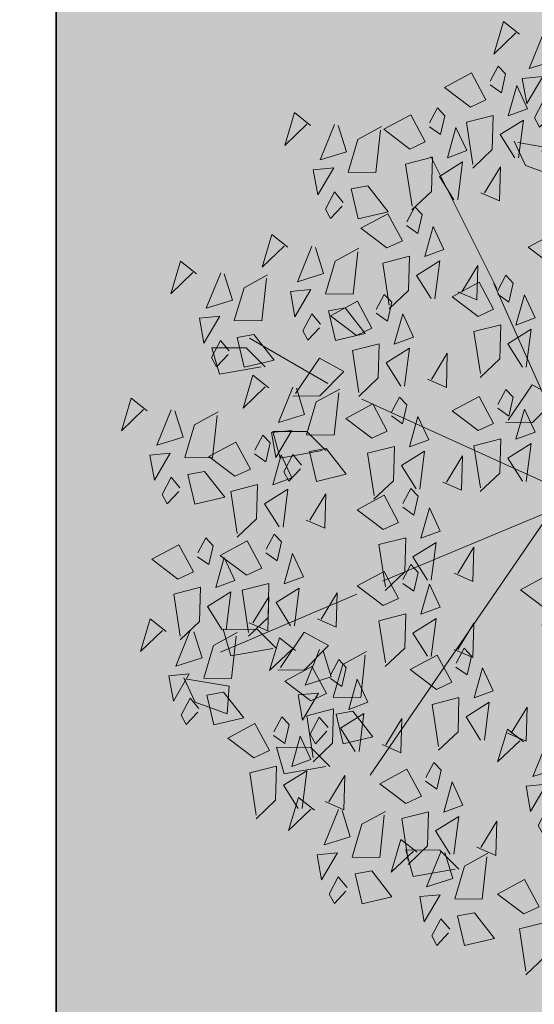
# Model space of a CAD drawing. Units: inches. Extents: x 1704 to 6393, y -157 to 1172.
# Tile 67 of 122: x 1897 to 1913, y 980 to 1010. Entities that reach past the tile are written whole.
import ezdxf

# ---------------------------------------------------------------- set-up
doc = ezdxf.new("R2010")
doc.units = ezdxf.units.IN
doc.header["$MEASUREMENT"] = 0
for name, color, linetype, lineweight in [('A-ANNO-DIMS', 7, 'Continuous', 13), ('C-PROP', 7, 'Continuous', 35), ('L-shrub', 74, 'Continuous', 18)]:
    doc.layers.add(name, color=color, linetype=linetype, lineweight=lineweight)
doc.layers.add('L-HRDS-PATT', color=9, linetype='Continuous', lineweight=13, true_color=0xc5c1ba)
doc.styles.get("Standard").update_dxf_attribs({"font": 'arial.ttf'})
doc.dimstyles.get("Standard").update_dxf_attribs({"dimtxt": 6, "dimasz": 2, "dimexe": 0.18, "dimexo": 0.0625, "dimgap": 0.09, "dimtad": 0, "dimtih": 1, "dimtoh": 1, "dimdec": 1, "dimzin": 0, "dimdsep": 46, "dimlunit": 3, "dimtxsty": 'Standard', "dimblk": 'ARCHTICK', "dimcen": 0.09, "dimadec": 0, "dimazin": 0, "dimtfac": 1, "dimtdec": 1, "dimtofl": 0, "dimtmove": 0, "dimatfit": 3, "dimfxl": 1, "dimtolj": 1, "dimtzin": 0, "dimarcsym": 0})

# ---------------------------------------------------------------- blocks, each defined once
blk = doc.blocks.new('flower shrub 3')
at = {"layer": 'L-shrub'}
for p, q in [((-123.45, 236), (-108.99, 242.75)), ((-109.76, 240.63), (-114.02, 215.74)), ((-130.41, 216.9), (-123.45, 236)), ((71.14, 221.55), (86.95, 226.01)), ((86.95, 226.01), (86.87, 205.67)), ((-114.02, 215.74), (-130.41, 216.9)), ((-96.02, 214.78), (-80.21, 219.24)), ((-80.21, 219.24), (-80.29, 198.91)), ((75.55, 196.68), (71.14, 221.55)), ((-91.61, 189.92), (-96.02, 214.78)), ((86.87, 205.67), (75.54, 194.43)), ((-80.29, 198.91), (-91.62, 187.66)), ((-166.05, 183.2), (-150.24, 187.65)), ((-150.24, 187.65), (-150.32, 167.32)), ((21.44, 185.45), (37.25, 189.91)), ((37.25, 189.91), (37.17, 169.58)), ((-161.64, 158.33), (-166.05, 183.2)), ((-104.33, 170.99), (-104.5, 186.95)), ((-102.88, 185.37), (-81.99, 171.19)), ((25.85, 160.59), (21.44, 185.45)), ((58.31, 161.96), (58.15, 177.93)), ((59.76, 176.34), (80.66, 162.16)), ((-89.82, 156.75), (-104.33, 170.99)), ((-81.99, 171.19), (-89.82, 156.75)), ((37.17, 169.58), (25.84, 158.33)), ((-150.32, 167.32), (-161.65, 156.07)), ((72.82, 147.73), (58.31, 161.96)), ((80.66, 162.16), (72.82, 147.73)), ((-227.04, 106.49), (-211.23, 110.94)), ((-222.63, 81.62), (-227.04, 106.49)), ((-211.23, 110.94), (-211.31, 90.61)), ((-211.31, 90.61), (-222.64, 79.36)), ((42.5, 35.62), (42.33, 51.58)), ((43.95, 50), (64.85, 35.82)), ((195.06, 39.71), (209.52, 46.47)), ((208.75, 44.35), (204.49, 19.45)), ((57.01, 21.38), (42.5, 35.62)), ((64.85, 35.82), (57.01, 21.38)), ((188.1, 20.61), (195.06, 39.71)), ((204.49, 19.45), (188.1, 20.61)), ((184.09, 9.47), (199.9, 13.93)), ((199.9, 13.93), (199.81, -6.4)), ((188.5, -15.39), (184.09, 9.47)), ((218.7, -20.78), (218.53, -4.82)), ((199.81, -6.4), (188.49, -17.65)), ((220.15, -6.4), (241.04, -20.58)), ((233.21, -35.02), (218.7, -20.78)), ((241.04, -20.58), (233.21, -35.02)), ((84.69, -53.7), (100.5, -49.25)), ((100.5, -49.25), (100.42, -69.58)), ((89.1, -78.57), (84.69, -53.7)), ((100.42, -69.58), (89.1, -80.83)), ((-205.99, -97.49), (-206.15, -81.53)), ((-204.54, -83.11), (-183.64, -97.29)), ((-191.47, -111.73), (-205.99, -97.49)), ((-183.64, -97.29), (-191.47, -111.73)), ((-161.53, -112.36), (-145.72, -107.91)), ((-145.72, -107.91), (-145.8, -128.24)), ((-157.12, -137.23), (-161.53, -112.36)), ((-179.93, -131.75), (-165.46, -125)), ((-166.23, -127.12), (-170.5, -152.01)), ((-145.8, -128.24), (-157.13, -139.49)), ((-186.88, -150.86), (-179.93, -131.75)), ((143.42, -141.69), (159.24, -137.24)), ((159.24, -137.24), (159.15, -157.57)), ((147.84, -166.56), (143.42, -141.69)), ((-170.5, -152.01), (-186.88, -150.86)), ((-163.07, -171.95), (-163.23, -155.98)), ((-161.62, -157.57), (-140.72, -171.75)), ((159.15, -157.57), (147.83, -168.82)), ((-148.55, -186.18), (-163.07, -171.95)), ((-140.72, -171.75), (-148.55, -186.18)), ((10.15, -195.84), (25.96, -191.38)), ((25.96, -191.38), (25.88, -211.71)), ((14.56, -220.7), (10.15, -195.84)), ((25.88, -211.71), (14.55, -222.96))]:
    blk.add_line(p, q, dxfattribs=at)
for points in [[(49.51, 264.41), (57.05, 273.94), (37.55, 279.71), (50.15, 266.57)], [(-81.5, 253.13), (-73.97, 262.66), (-93.47, 268.43), (-80.86, 255.29)], [(-50.38, 246.16), (-38.67, 261.64), (-30.06, 245.61), (-46.11, 237.01), (-50.38, 246.16)], [(24.26, 250.7), (23.13, 262.8), (8.21, 260.16), (24.26, 250.7)], [(49.36, 247.98), (33.81, 243.17), (28.98, 258.72), (50, 250.14)], [(-106.76, 239.42), (-107.89, 251.52), (-122.81, 248.88), (-106.76, 239.42)], [(3.73, 245.02), (9.98, 250.22), (-0.21, 255.59), (-5.82, 252.55), (1.56, 245.66)], [(-81.65, 236.7), (-97.21, 231.89), (-102.03, 247.44), (-81.01, 238.86)], [(-84.31, 244.82), (-59.35, 248.66), (-55.26, 232.75), (-75.59, 233.29), (-86.57, 244.88)], [(130.84, 235.08), (138.37, 244.61), (118.87, 250.38), (131.48, 237.24)], [(-127.29, 233.74), (-121.04, 238.94), (-131.23, 244.31), (-136.84, 241.27), (-129.46, 234.38)], [(13.52, 230.35), (-1.79, 218.41), (-5.97, 236.12), (11.75, 240.29), (13.52, 230.35)], [(46.65, 222.9), (21.55, 225.63), (21.7, 242.05), (41.19, 236.28), (48.82, 222.26)], [(-37.14, 234.51), (-41.84, 227.87), (-30.61, 225.31), (-25.97, 229.7), (-34.88, 234.45)], [(-117.5, 219.07), (-132.81, 207.13), (-136.99, 224.84), (-119.27, 229.01), (-117.5, 219.07)], [(-84.36, 211.62), (-109.47, 214.34), (-109.32, 230.77), (-89.83, 225), (-82.2, 210.98)], [(-80.47, 219.88), (-66.68, 228.54), (-58.01, 214.76), (-80.53, 217.63)], [(105.58, 221.37), (104.45, 233.47), (89.53, 230.83), (105.58, 221.37)], [(130.69, 218.65), (115.13, 213.84), (110.31, 229.39), (131.33, 220.81)], [(-55.51, 223.72), (-51.3, 212.33), (-37.56, 218.73), (-55.51, 223.72)], [(10.61, 212.31), (22.33, 227.8), (30.93, 211.77), (14.88, 203.17), (10.61, 212.31)], [(85.05, 215.69), (91.3, 220.89), (81.11, 226.26), (75.5, 223.22), (82.88, 216.33)], [(-156.55, 201.03), (-144.84, 216.52), (-136.23, 200.48), (-152.28, 191.89), (-156.55, 201.03)], [(-59.39, 140.01), (-93.72, 220.83)], [(-48.12, 205.55), (-36.41, 221.03), (-27.8, 205), (-43.85, 196.4), (-48.12, 205.55)], [(-23.32, 210.97), (1.64, 214.81), (5.73, 198.9), (-14.6, 199.45), (-25.58, 211.03)], [(94.84, 201.02), (79.53, 189.08), (75.35, 206.79), (93.07, 210.96), (94.84, 201.02)], [(127.98, 193.57), (102.87, 196.3), (103.02, 212.72), (122.51, 206.95), (130.14, 192.93)], [(-82.06, 204.2), (-57.09, 208.04), (-53, 192.14), (-73.33, 192.68), (-84.31, 204.27)], [(63.07, 192.21), (70.6, 201.74), (51.11, 207.51), (63.71, 194.37)], [(-190.49, 199.69), (-165.52, 203.53), (-161.43, 187.62), (-181.76, 188.17), (-192.74, 199.75)], [(-76.38, 203.98), (-81.2, 192.82), (-60.88, 192.27), (-76.44, 201.72)], [(23.85, 200.67), (19.16, 194.03), (30.38, 191.47), (35.02, 195.86), (26.11, 200.61)], [(65.66, 157.16), (92.63, 203.69)], [(-34.88, 193.9), (-39.58, 187.26), (-28.35, 184.7), (-23.71, 189.09), (-32.62, 193.84)], [(-19.48, 186.04), (-5.68, 194.7), (2.98, 180.92), (-19.54, 183.79)], [(146.65, 180.93), (154.18, 190.46), (134.69, 196.23), (147.29, 183.09)], [(-143.31, 189.39), (-148.01, 182.75), (-136.78, 180.19), (-132.14, 184.58), (-141.05, 189.33)], [(-92.8, 176.42), (-85.27, 185.95), (-104.76, 191.72), (-92.16, 178.58)], [(-78.21, 179.27), (-64.42, 187.93), (-55.75, 174.15), (-78.27, 177.02)], [(5.48, 189.88), (9.7, 178.48), (23.43, 184.88), (5.48, 189.88)], [(37.81, 178.51), (36.68, 190.61), (21.76, 187.96), (37.81, 178.51)], [(-186.64, 174.76), (-172.85, 183.42), (-164.18, 169.64), (-186.7, 172.51)], [(-122.67, 167.19), (-110.95, 182.67), (-102.35, 166.64), (-118.4, 158.05), (-122.67, 167.19)], [(-53.25, 183.11), (-49.04, 171.72), (-35.3, 178.12), (-53.25, 183.11)], [(17.28, 172.82), (23.53, 178.03), (13.34, 183.4), (7.73, 180.35), (15.12, 173.46)], [(62.92, 175.78), (47.36, 170.98), (42.54, 186.52), (63.56, 177.95)], [(218.93, 167.39), (226.47, 176.93), (206.97, 182.7), (219.58, 169.56)], [(-187.68, 165.14), (-180.14, 174.67), (-199.64, 180.44), (-187.04, 167.3)], [(-161.68, 178.6), (-157.47, 167.2), (-143.73, 173.6), (-161.68, 178.6)], [(121.39, 167.23), (120.26, 179.33), (105.34, 176.68), (121.39, 167.23)], [(-156.6, 165.85), (-131.64, 169.69), (-127.55, 153.78), (-147.87, 154.33), (-158.86, 165.91)], [(-118.06, 162.71), (-119.19, 174.81), (-134.1, 172.17), (-118.06, 162.71)], [(-92.95, 159.99), (-108.51, 155.18), (-113.33, 170.73), (-92.31, 162.15)], [(-15.39, 170.13), (-20.21, 158.98), (0.12, 158.43), (-15.45, 167.88)], [(60.21, 150.7), (35.1, 153.43), (35.25, 169.85), (54.74, 164.09), (62.37, 150.06)], [(100.86, 161.54), (107.11, 166.75), (96.92, 172.11), (91.31, 169.07), (98.7, 162.18)], [(146.5, 164.5), (130.94, 159.7), (126.12, 175.24), (147.14, 166.67)], [(-138.59, 157.03), (-132.33, 162.23), (-142.52, 167.6), (-148.14, 164.56), (-140.75, 157.67)], [(27.08, 158.16), (11.76, 146.22), (7.58, 163.93), (25.31, 168.09), (27.08, 158.16)], [(193.68, 153.69), (192.55, 165.79), (177.63, 163.15), (193.68, 153.69)], [(-212.93, 151.43), (-214.06, 163.53), (-228.98, 160.89), (-212.93, 151.43)], [(-187.82, 148.71), (-203.38, 143.9), (-208.21, 159.45), (-187.18, 150.87)], [(-182.55, 158.85), (-187.37, 147.7), (-167.05, 147.15), (-182.61, 156.6)], [(-74.12, 163.36), (-78.94, 152.21), (-58.62, 151.66), (-74.18, 161.11)], [(143.79, 139.42), (118.68, 142.15), (118.83, 158.57), (138.33, 152.8), (145.96, 138.78)], [(173.15, 148), (179.4, 153.21), (169.21, 158.58), (163.6, 155.53), (170.98, 148.64)], [(218.79, 150.97), (203.23, 146.16), (198.41, 161.7), (219.43, 153.13)], [(-233.46, 145.75), (-227.21, 150.95), (-237.4, 156.32), (-243.01, 153.28), (-235.63, 146.39)], [(-128.79, 142.36), (-144.1, 130.42), (-148.29, 148.13), (-130.56, 152.3), (-128.79, 142.36)], [(-95.66, 134.91), (-120.77, 137.64), (-120.62, 154.06), (-101.12, 148.29), (-93.49, 134.27)], [(-109.42, 155.55), (-114.12, 148.9), (-102.89, 146.34), (-98.26, 150.73), (-107.17, 155.49)], [(110.66, 146.88), (95.35, 134.94), (91.16, 152.64), (108.89, 156.81), (110.66, 146.88)], [(94.19, 140.12), (105.91, 155.6), (114.51, 139.57), (98.46, 130.97), (94.19, 140.12)], [(-152.75, 140.92), (-138.96, 149.57), (-130.29, 135.8), (-152.82, 138.66)], [(33.2, 131.09), (44.92, 146.57), (53.52, 130.54), (37.47, 121.95), (33.2, 131.09)], [(-223.67, 131.08), (-238.98, 119.14), (-243.16, 136.85), (-225.44, 141.02), (-223.67, 131.08)], [(-190.53, 123.63), (-215.64, 126.35), (-215.49, 142.78), (-196, 137.01), (-188.37, 122.99)], [(-127.79, 144.76), (-123.58, 133.36), (-109.85, 139.76), (-127.79, 144.76)], [(60.26, 138.78), (85.22, 142.62), (89.31, 126.71), (68.99, 127.26), (58, 138.84)], [(182.94, 133.34), (167.63, 121.4), (163.45, 139.11), (181.17, 143.27), (182.94, 133.34)], [(216.08, 125.89), (190.97, 128.61), (191.12, 145.04), (210.61, 139.27), (218.24, 125.25)], [(-66.19, 124.32), (-54.48, 139.81), (-45.87, 123.78), (-61.92, 115.18), (-66.19, 124.32)], [(-21.02, 124.32), (-9.3, 139.81), (-0.69, 123.78), (-16.74, 115.18), (-21.02, 124.32)], [(-2.54, 7.13), (56.31, 136.92)], [(146.15, 122.07), (157.86, 137.55), (166.47, 121.52), (150.42, 112.92), (146.15, 122.07)], [(-9.89, 24.27), (-166.82, 132.02)], [(-0.73, 129.75), (24.23, 133.59), (28.32, 117.68), (7.99, 118.23), (-2.99, 129.81)], [(-183.66, 110.79), (-171.94, 126.27), (-163.34, 110.24), (-179.39, 101.64), (-183.66, 110.79)], [(-148.66, 125.01), (-153.48, 113.86), (-133.16, 113.31), (-148.73, 122.75)], [(-100.13, 122.98), (-75.17, 126.82), (-71.08, 110.91), (-91.4, 111.46), (-102.39, 123.04)], [(-54.95, 122.98), (-29.99, 126.82), (-25.9, 110.91), (-46.22, 111.46), (-57.21, 123.04)], [(-2.54, 7.13), (-51.58, 124.68)], [(107.43, 128.47), (102.74, 121.83), (113.97, 119.27), (118.6, 123.66), (109.69, 128.41)], [(112.21, 120.73), (137.17, 124.57), (141.26, 108.66), (120.94, 109.21), (109.96, 120.79)], [(204.88, 108.53), (216.6, 124.01), (225.2, 107.98), (209.15, 99.39), (204.88, 108.53)], [(-212.52, 104.22), (-204.99, 113.75), (-224.49, 119.52), (-211.88, 106.38)], [(46.44, 119.45), (41.74, 112.81), (52.97, 110.25), (57.61, 114.63), (48.7, 119.39)], [(64.1, 113.85), (77.9, 122.5), (86.56, 108.73), (64.04, 111.59)], [(89.07, 117.69), (93.28, 106.29), (107.01, 112.69), (89.07, 117.69)], [(-217.59, 109.45), (-192.63, 113.29), (-188.54, 97.38), (-208.86, 97.93), (-219.85, 109.51)], [(-52.95, 112.68), (-57.65, 106.04), (-46.42, 103.48), (-41.78, 107.87), (-50.69, 112.62)], [(-7.77, 112.68), (-12.47, 106.04), (-1.24, 103.48), (3.4, 107.87), (-5.51, 112.62)], [(3.11, 104.82), (16.91, 113.48), (25.57, 99.7), (3.05, 102.57)], [(-115.89, 92.74), (-104.17, 108.22), (-95.57, 92.19), (-111.62, 83.59), (-115.89, 92.74)], [(-96.28, 98.05), (-82.49, 106.71), (-73.82, 92.93), (-96.34, 95.8)], [(-51.1, 98.05), (-37.31, 106.71), (-28.64, 92.93), (-51.16, 95.8)], [(28.07, 108.66), (32.29, 97.26), (46.02, 103.66), (28.07, 108.66)], [(159.39, 110.43), (154.69, 103.78), (165.92, 101.22), (170.56, 105.61), (161.65, 110.36)], [(170.95, 107.19), (195.91, 111.03), (200, 95.12), (179.67, 95.67), (168.69, 107.25)], [(-237.78, 90.52), (-238.91, 102.62), (-253.83, 99.97), (-237.78, 90.52)], [(-71.32, 101.89), (-67.11, 90.49), (-53.38, 96.89), (-71.32, 101.89)], [(-26.14, 101.89), (-21.93, 90.49), (-8.2, 96.89), (-26.14, 101.89)], [(116.06, 95.8), (129.85, 104.45), (138.52, 90.68), (116, 93.54)], [(141.02, 99.64), (145.23, 88.24), (158.96, 94.64), (141.02, 99.64)], [(-258.31, 84.83), (-252.06, 90.04), (-262.25, 95.41), (-267.86, 92.36), (-260.48, 85.47)], [(-212.67, 87.79), (-228.23, 82.99), (-233.05, 98.53), (-212.03, 89.96)], [(-170.42, 99.14), (-175.11, 92.5), (-163.88, 89.94), (-159.25, 94.33), (-168.16, 99.08)], [(-149.82, 91.4), (-124.86, 95.24), (-120.77, 79.33), (-141.1, 79.88), (-152.08, 91.46)], [(68.19, 97.94), (63.37, 86.78), (83.7, 86.23), (68.13, 95.68)], [(122.05, 56.75), (200.52, 95.93)], [(218.12, 96.89), (213.42, 90.24), (224.65, 87.68), (229.29, 92.07), (220.38, 96.83)], [(-213.75, 84.52), (-199.95, 93.17), (-191.29, 79.4), (-213.81, 82.26)], [(-188.78, 88.36), (-184.57, 76.96), (-170.84, 83.36), (-188.78, 88.36)], [(7.2, 88.91), (2.38, 77.76), (22.71, 77.21), (7.14, 86.66)], [(174.79, 82.26), (188.58, 90.91), (197.25, 77.14), (174.73, 80)], [(229.73, 72.43), (241.44, 87.91), (250.05, 71.88), (234, 63.29), (229.73, 72.43)], [(-215.38, 62.71), (-240.49, 65.44), (-240.34, 81.86), (-220.85, 76.1), (-213.22, 62.07)], [(-92.19, 82.14), (-97.01, 70.99), (-76.69, 70.44), (-92.25, 79.89)], [(-47.01, 82.14), (-51.83, 70.99), (-31.51, 70.44), (-47.07, 79.89)], [(37.72, 67.92), (49.43, 83.4), (58.04, 67.37), (41.99, 58.78), (37.72, 67.92)], [(105.49, 67.92), (117.2, 83.4), (125.81, 67.37), (109.76, 58.78), (105.49, 67.92)], [(199.75, 86.1), (203.97, 74.7), (217.7, 81.1), (199.75, 86.1)], [(-248.51, 70.17), (-263.83, 58.23), (-268.01, 75.94), (-250.29, 80.1), (-248.51, 70.17)], [(-102.65, 81.1), (-107.35, 74.45), (-96.12, 71.89), (-91.48, 76.28), (-100.39, 81.03)], [(120.15, 79.89), (115.33, 68.73), (135.65, 68.18), (120.09, 77.63)], [(-145.98, 66.47), (-132.19, 75.12), (-123.52, 61.35), (-146.04, 64.21)], [(-121.02, 70.31), (-116.8, 58.91), (-103.07, 65.31), (-121.02, 70.31)], [(3.78, 66.58), (28.75, 70.42), (32.84, 54.51), (12.51, 55.06), (1.53, 66.64)], [(71.55, 66.58), (96.51, 70.42), (100.6, 54.51), (80.28, 55.06), (69.29, 66.64)], [(195.79, 71.09), (220.76, 74.93), (224.85, 59.02), (204.52, 59.57), (193.54, 71.15)], [(-209.66, 68.61), (-214.48, 57.45), (-194.15, 56.9), (-209.72, 66.35)], [(178.88, 66.35), (174.06, 55.2), (194.39, 54.65), (178.82, 64.09)], [(9.72, 7.13), (124.97, 58.56)], [(242.97, 60.79), (238.27, 54.15), (249.5, 51.59), (254.14, 55.97), (245.23, 60.73)], [(273.15, 43.3), (280.68, 52.84), (261.19, 58.61), (273.79, 45.47)], [(-249.17, 40.85), (-237.45, 56.33), (-228.85, 40.3), (-244.9, 31.7), (-249.17, 40.85)], [(-147.01, 41.05), (-139.48, 50.58), (-158.98, 56.35), (-146.37, 43.21)], [(50.96, 56.28), (46.26, 49.63), (57.49, 47.07), (62.13, 51.46), (53.22, 56.22)], [(118.73, 56.28), (114.03, 49.63), (125.26, 47.07), (129.9, 51.46), (120.99, 56.22)], [(199.64, 46.16), (213.43, 54.82), (222.1, 41.04), (199.58, 43.91)], [(-141.89, 50.56), (-146.71, 39.4), (-126.38, 38.85), (-141.95, 48.3)], [(7.63, 41.65), (21.42, 50.3), (30.09, 36.53), (7.57, 39.39)], [(75.4, 41.65), (89.19, 50.3), (97.86, 36.53), (75.34, 39.39)], [(224.6, 50), (228.81, 38.6), (242.55, 45), (224.6, 50)], [(-283.1, 39.51), (-258.14, 43.35), (-254.05, 27.44), (-274.37, 27.98), (-285.36, 39.57)], [(-68.45, 27.31), (-56.74, 42.79), (-48.13, 26.76), (-64.18, 18.17), (-68.45, 27.31)], [(32.59, 45.49), (36.8, 34.09), (50.54, 40.49), (32.59, 45.49)], [(100.36, 45.49), (104.57, 34.09), (118.3, 40.49), (100.36, 45.49)], [(247.89, 29.6), (246.76, 41.7), (231.84, 39.06), (247.89, 29.6)], [(-172.27, 27.35), (-173.4, 39.44), (-188.32, 36.8), (-172.27, 27.35)], [(-147.16, 24.62), (-162.72, 19.81), (-167.54, 35.36), (-146.52, 26.78)], [(134.85, 22.8), (146.57, 38.28), (155.17, 22.25), (139.12, 13.65), (134.85, 22.8)], [(273, 26.88), (257.44, 22.07), (252.62, 37.61), (273.64, 29.04)], [(-192.8, 21.66), (-186.55, 26.86), (-196.74, 32.23), (-202.35, 29.19), (-194.97, 22.3)], [(-102.39, 25.97), (-77.43, 29.81), (-73.34, 13.9), (-93.66, 14.45), (-104.64, 26.03)], [(203.73, 30.25), (198.91, 19.1), (219.23, 18.55), (203.67, 28)], [(227.36, 23.91), (233.62, 29.12), (223.43, 34.49), (217.81, 31.44), (225.2, 24.55)], [(-235.92, 29.2), (-240.62, 22.56), (-229.39, 20), (-224.76, 24.39), (-233.67, 29.14)], [(11.72, 25.74), (6.9, 14.58), (27.22, 14.04), (11.66, 23.48)], [(14.63, 7.13), (137.23, 26.72)], [(79.49, 25.74), (74.67, 14.58), (94.99, 14.04), (79.43, 23.48)], [(100.92, 21.46), (125.88, 25.3), (129.97, 9.39), (109.65, 9.94), (98.66, 21.52)], [(-279.26, 14.57), (-265.46, 23.23), (-256.8, 9.45), (-279.32, 12.32)], [(-254.29, 18.41), (-250.08, 7.02), (-236.35, 13.42), (-254.29, 18.41)], [(-149.87, -0.46), (-174.98, 2.27), (-174.83, 18.69), (-155.34, 12.92), (-147.71, -1.1)], [(-113.13, 7.2), (-105.6, 16.74), (-125.09, 22.51), (-112.49, 9.37)], [(92.43, 4.95), (99.97, 14.48), (80.47, 20.25), (93.07, 7.11)], [(237.16, 9.25), (221.85, -2.69), (217.66, 15.02), (235.39, 19.19), (237.16, 9.25)], [(270.29, 1.8), (245.18, 4.52), (245.33, 20.95), (264.83, 15.18), (272.46, 1.16)], [(-183.01, 6.99), (-198.32, -4.95), (-202.5, 12.76), (-184.78, 16.93), (-183.01, 6.99)], [(-138.39, -6.5), (-139.52, 5.6), (-154.26, 11.88), (-138.39, -6.5)], [(-55.21, 15.67), (-59.91, 9.02), (-48.68, 6.46), (-44.04, 10.85), (-52.95, 15.61)], [(168.74, 0.24), (180.45, 15.72), (189.06, -0.31), (173.01, -8.91), (168.74, 0.24)], [(-98.54, 1.04), (-84.75, 9.69), (-76.08, -4.08), (-98.6, -1.22)], [(148.1, 11.15), (143.4, 4.51), (154.63, 1.95), (159.26, 6.34), (150.35, 11.09)], [(-7.44, 4.68), (-201.15, -54.09)], [(-113.28, -9.22), (-128.84, -14.03), (-133.66, 1.52), (-112.64, -7.06)], [(-73.58, 4.88), (-69.37, -6.52), (-55.64, -0.12), (-73.58, 4.88)], [(14.63, 4.68), (156.84, -137.36)], [(67.18, -8.75), (66.05, 3.35), (51.13, 0.7), (67.18, -8.75)], [(104.77, -3.47), (118.56, 5.18), (127.22, -8.59), (104.7, -5.73)], [(129.73, 0.37), (133.94, -11.03), (147.67, -4.63), (129.73, 0.37)], [(134.8, -1.11), (159.76, 2.73), (163.85, -13.17), (143.53, -12.63), (132.54, -1.04)], [(-275.17, -1.33), (-279.99, -12.49), (-259.66, -13.04), (-275.23, -3.59)], [(-197.21, -15.56), (-185.5, -0.08), (-176.89, -16.11), (-192.94, -24.7), (-197.21, -15.56)], [(-2.54, -0.22), (-181.53, -98.18)], [(-158.92, -12.19), (-152.66, -6.98), (-162.85, -1.61), (-168.47, -4.65), (-161.08, -11.54)], [(-2.54, -5.12), (-51.58, -205.93)], [(-41.35, -15.56), (-29.63, -0.08), (-21.02, -16.11), (-37.07, -24.7), (-41.35, -15.56)], [(46.65, -14.44), (52.9, -9.23), (42.71, -3.87), (37.1, -6.91), (44.48, -13.8)], [(92.28, -11.48), (76.73, -16.28), (71.9, -0.74), (92.92, -9.31)], [(7.27, -10.01), (132.32, -196.13)], [(181.98, -11.41), (177.28, -18.05), (188.51, -20.61), (193.15, -16.22), (184.24, -11.47)], [(223.45, -26.64), (230.99, -17.1), (211.49, -11.33), (224.09, -24.47)], [(-231.15, -16.9), (-206.18, -13.06), (-202.09, -28.97), (-222.42, -28.42), (-233.4, -16.84)], [(-149.12, -26.85), (-164.43, -38.79), (-168.62, -21.08), (-150.89, -16.91), (-149.12, -26.85)], [(-115.99, -34.3), (-141.1, -31.58), (-140.95, -15.15), (-121.45, -20.92), (-113.82, -34.94)], [(-94.45, -14.87), (-99.27, -26.03), (-78.95, -26.58), (-94.51, -17.13)], [(-75.28, -16.9), (-50.32, -13.06), (-46.23, -28.97), (-66.55, -28.42), (-77.54, -16.84)], [(89.57, -36.56), (64.47, -33.83), (64.62, -17.41), (84.11, -23.18), (91.74, -37.2)], [(138.65, -26.04), (152.44, -17.38), (161.11, -31.16), (138.59, -28.29)], [(56.44, -29.1), (41.13, -41.04), (36.95, -23.34), (54.67, -19.17), (56.44, -29.1)], [(108.86, -19.38), (104.03, -30.54), (124.36, -31.09), (108.79, -21.64)], [(163.61, -22.2), (167.82, -33.59), (181.55, -27.19), (163.61, -22.2)], [(-183.97, -27.2), (-188.67, -33.84), (-177.44, -36.4), (-172.8, -32.02), (-181.71, -27.26)], [(-28.1, -27.2), (-32.8, -33.84), (-21.57, -36.4), (-16.93, -32.02), (-25.84, -27.26)], [(55.85, -28.96), (171.09, -41.21)], [(198.2, -40.34), (197.06, -28.24), (182.15, -30.88), (198.2, -40.34)], [(-227.3, -41.83), (-213.51, -33.17), (-204.84, -46.95), (-227.36, -44.08)], [(-71.43, -41.83), (-57.64, -33.17), (-48.97, -46.95), (-71.49, -44.08)], [(37.72, -47.14), (49.43, -31.66), (58.04, -47.69), (41.99, -56.29), (37.72, -47.14)], [(223.3, -43.06), (207.75, -47.87), (202.92, -32.33), (223.94, -40.9)], [(-202.34, -37.99), (-198.13, -49.39), (-184.4, -42.99), (-202.34, -37.99)], [(-124.93, -51.66), (-113.21, -36.17), (-104.6, -52.2), (-120.65, -60.8), (-124.93, -51.66)], [(-46.47, -37.99), (-42.26, -49.39), (-28.53, -42.99), (-46.47, -37.99)], [(-18.76, -53.91), (-7.04, -38.43), (1.57, -54.46), (-14.48, -63.06), (-18.76, -53.91)], [(119.54, -51.46), (127.07, -41.92), (107.58, -36.15), (120.18, -49.29)], [(177.67, -46.03), (183.92, -40.82), (173.73, -35.45), (168.12, -38.5), (175.5, -45.39)], [(-151.53, -58.22), (-144, -48.69), (-163.49, -42.92), (-150.89, -56.06)], [(3.78, -48.48), (28.75, -44.64), (32.84, -60.55), (12.51, -60.01), (1.53, -48.42)], [(142.74, -41.95), (137.92, -53.1), (158.24, -53.65), (142.68, -44.2)], [(-158.86, -53), (-133.9, -49.16), (-129.81, -65.07), (-150.13, -64.52), (-161.12, -52.94)], [(-52.69, -55.25), (-27.73, -51.41), (-23.64, -67.32), (-43.96, -66.77), (-54.95, -55.19)], [(187.46, -60.69), (172.15, -72.63), (167.97, -54.92), (185.69, -50.76), (187.46, -60.69)], [(220.59, -68.14), (195.49, -65.42), (195.64, -48.99), (215.13, -54.76), (222.76, -68.78)], [(266.37, -67.25), (273.91, -57.71), (254.41, -51.94), (267.01, -65.08)], [(-223.21, -57.74), (-228.03, -68.89), (-207.71, -69.44), (-223.27, -59.99)], [(-67.34, -57.74), (-72.16, -68.89), (-51.84, -69.44), (-67.4, -59.99)], [(94.28, -65.16), (93.15, -53.06), (78.24, -55.7), (94.28, -65.16)], [(119.39, -67.88), (103.83, -72.69), (99.01, -57.14), (120.03, -65.72)], [(204.88, -69.71), (216.6, -54.22), (225.2, -70.25), (209.15, -78.85), (204.88, -69.71)], [(-176.79, -71.93), (-177.92, -59.83), (-192.84, -62.47), (-176.79, -71.93)], [(-151.68, -74.65), (-167.24, -79.46), (-172.06, -63.91), (-151.04, -72.49)], [(-111.68, -63.3), (-116.38, -69.94), (-105.15, -72.5), (-100.51, -68.11), (-109.42, -63.36)], [(50.96, -58.79), (46.26, -65.43), (57.49, -67.99), (62.13, -63.6), (53.22, -58.85)], [(73.75, -70.85), (80.01, -65.64), (69.82, -60.27), (64.2, -63.31), (71.59, -70.2)], [(-197.32, -77.61), (-191.07, -72.41), (-201.26, -67.04), (-206.87, -70.08), (-199.48, -76.97)], [(-155.01, -77.93), (-141.22, -69.27), (-132.55, -83.05), (-155.07, -80.18)], [(-5.51, -65.55), (-10.21, -72.2), (1.02, -74.76), (5.66, -70.37), (-3.25, -65.62)], [(7.63, -73.42), (21.42, -64.76), (30.09, -78.54), (7.57, -75.67)], [(32.59, -69.58), (36.8, -80.97), (50.54, -74.57), (32.59, -69.58)], [(170.95, -71.05), (195.91, -67.21), (200, -83.12), (179.67, -82.57), (168.69, -70.99)], [(241.12, -80.95), (239.98, -68.85), (225.07, -71.49), (241.12, -80.95)], [(-130.05, -74.09), (-125.84, -85.49), (-112.11, -79.09), (-130.05, -74.09)], [(-115.89, -90.01), (-104.17, -74.53), (-95.57, -90.56), (-111.62, -99.15), (-115.89, -90.01)], [(-48.84, -80.18), (-35.05, -71.53), (-26.38, -85.3), (-48.9, -82.44)], [(83.55, -85.51), (68.24, -97.45), (64.06, -79.74), (81.78, -75.57), (83.55, -85.51)], [(116.68, -92.96), (91.57, -90.24), (91.72, -73.81), (111.22, -79.58), (118.85, -93.6)], [(116.78, -90.01), (128.5, -74.53), (137.1, -90.56), (121.05, -99.15), (116.78, -90.01)], [(266.22, -83.67), (250.67, -88.48), (245.84, -72.94), (266.86, -81.51)], [(-154.39, -99.73), (-179.5, -97), (-179.35, -80.58), (-159.85, -86.35), (-152.23, -100.37)], [(-49.88, -94.32), (-42.35, -84.79), (-61.84, -79.02), (-49.24, -92.16)], [(-23.88, -76.34), (-19.67, -87.74), (-5.94, -81.34), (-23.88, -76.34)], [(220.59, -86.64), (226.84, -81.43), (216.65, -76.06), (211.04, -79.11), (218.42, -86)], [(218.12, -81.35), (213.42, -87.99), (224.65, -90.55), (229.29, -86.16), (220.38, -81.41)], [(-196.71, -101.09), (-189.18, -91.56), (-208.67, -85.79), (-196.07, -98.93)], [(-187.52, -92.28), (-202.84, -104.22), (-207.02, -86.51), (-189.29, -82.34), (-187.52, -92.28)], [(-149.82, -91.35), (-124.86, -87.51), (-120.77, -103.42), (-141.1, -102.87), (-152.08, -91.29)], [(82.85, -91.35), (107.81, -87.51), (111.9, -103.42), (91.58, -102.87), (80.59, -91.29)], [(174.79, -95.98), (188.58, -87.32), (197.25, -101.1), (174.73, -98.23)], [(-12.8, -148.96), (-20.16, -90.19)], [(11.72, -89.32), (6.9, -100.48), (27.22, -101.03), (11.66, -91.58)], [(62.57, -103.55), (74.28, -88.07), (82.89, -104.1), (66.84, -112.69), (62.57, -103.55)], [(199.75, -92.14), (203.97, -103.54), (217.7, -97.14), (199.75, -92.14)], [(230.38, -101.3), (215.07, -113.24), (210.89, -95.53), (228.61, -91.37), (230.38, -101.3)], [(263.51, -108.75), (238.41, -106.03), (238.56, -89.6), (258.05, -95.37), (265.68, -109.39)], [(-150.92, -93.84), (-155.74, -104.99), (-135.42, -105.54), (-150.98, -96.09)], [(-75.14, -108.02), (-76.27, -95.92), (-91.18, -98.57), (-75.14, -108.02)], [(-44.75, -96.09), (-49.57, -107.25), (-29.25, -107.8), (-44.81, -98.35)], [(-221.97, -114.79), (-223.1, -102.69), (-238.02, -105.34), (-221.97, -114.79)], [(-102.65, -101.65), (-107.35, -108.3), (-96.12, -110.86), (-91.48, -106.47), (-100.39, -101.71)], [(-95.67, -113.71), (-89.41, -108.5), (-99.6, -103.14), (-105.22, -106.18), (-97.83, -113.07)], [(-50.03, -110.75), (-65.59, -115.56), (-70.41, -100.01), (-49.39, -108.58)], [(28.63, -104.89), (53.59, -101.05), (57.68, -116.96), (37.36, -116.41), (26.37, -104.83)], [(70.56, -104.88), (75.47, -144.06)], [(130.02, -101.65), (125.33, -108.3), (136.56, -110.86), (141.19, -106.47), (132.28, -101.71)], [(182.29, -117.08), (194.01, -101.6), (202.61, -117.63), (186.56, -126.23), (182.29, -117.08)], [(-242.5, -120.48), (-236.24, -115.27), (-246.44, -109.9), (-252.05, -112.95), (-244.66, -119.84)], [(-196.86, -117.52), (-212.42, -122.32), (-217.24, -106.78), (-196.22, -115.35)], [(-145.98, -116.28), (-132.19, -107.63), (-123.52, -121.4), (-146.04, -118.54)], [(86.69, -116.28), (100.49, -107.63), (109.15, -121.4), (86.63, -118.54)], [(-121.02, -112.44), (-116.8, -123.84), (-103.07, -117.44), (-121.02, -112.44)], [(-52.74, -135.83), (-77.85, -133.1), (-77.7, -116.68), (-58.2, -122.45), (-50.57, -136.47)], [(75.81, -115.19), (71.11, -121.83), (82.34, -124.39), (86.98, -120.01), (78.07, -115.25)], [(111.65, -112.44), (115.87, -123.84), (129.6, -117.44), (111.65, -112.44)], [(148.36, -118.43), (173.32, -114.59), (177.41, -130.49), (157.08, -129.95), (146.1, -118.36)], [(178.88, -111.89), (174.06, -123.04), (194.39, -123.59), (178.82, -114.14)], [(-181.4, -137.39), (-169.68, -121.91), (-161.08, -137.94), (-177.13, -146.53), (-181.4, -137.39)], [(-85.87, -128.38), (-101.18, -140.31), (-105.37, -122.61), (-87.64, -118.44), (-85.87, -128.38)], [(-0.69, -135.13), (11.03, -119.65), (19.64, -135.68), (3.59, -144.28), (-0.69, -135.13)], [(32.48, -129.82), (46.27, -121.16), (54.94, -134.94), (32.42, -132.07)], [(151.17, -134.93), (158.7, -125.4), (139.2, -119.63), (151.81, -132.77)], [(-232.7, -135.14), (-248.01, -147.08), (-252.2, -129.38), (-234.47, -125.21), (-232.7, -135.14)], [(-199.57, -142.6), (-224.68, -139.87), (-224.53, -123.45), (-205.03, -129.21), (-197.4, -143.24)], [(57.44, -125.98), (61.65, -137.38), (75.38, -130.98), (57.44, -125.98)], [(-141.89, -132.19), (-146.71, -143.35), (-126.38, -143.9), (-141.95, -134.45)], [(-63.94, -146.41), (-52.22, -130.93), (-43.61, -146.96), (-59.66, -155.56), (-63.94, -146.41)], [(-34.62, -136.47), (-9.66, -132.63), (-5.57, -148.54), (-25.89, -148), (-36.88, -136.41)], [(90.78, -132.19), (85.96, -143.35), (106.29, -143.9), (90.72, -134.45)], [(195.53, -128.73), (190.83, -135.37), (202.06, -137.93), (206.7, -133.54), (197.79, -128.79)], [(-215.33, -138.73), (-190.37, -134.89), (-186.28, -150.8), (-206.61, -150.25), (-217.59, -138.67)], [(125.91, -148.63), (124.78, -136.54), (109.86, -139.18), (125.91, -148.63)], [(152.2, -143.36), (166, -134.7), (174.66, -148.48), (152.14, -145.61)], [(177.16, -139.52), (181.38, -150.91), (195.11, -144.51), (177.16, -139.52)], [(-97.87, -147.76), (-72.91, -143.92), (-68.82, -159.82), (-89.14, -159.28), (-100.13, -147.69)], [(36.57, -145.73), (31.75, -156.88), (52.07, -157.43), (36.51, -147.98)], [(105.38, -154.32), (111.63, -149.12), (101.44, -143.75), (95.83, -146.79), (103.21, -153.68)], [(151.02, -151.36), (135.46, -156.17), (130.64, -140.62), (151.66, -149.2)], [(-168.16, -149.03), (-172.86, -155.68), (-161.63, -158.24), (-156.99, -153.85), (-165.9, -149.09)], [(-12.34, -147.15), (-0.08, -242.66)], [(12.56, -146.78), (7.86, -153.42), (19.09, -155.98), (23.73, -151.59), (14.82, -146.84)], [(-211.49, -163.66), (-197.69, -155.01), (-189.03, -168.78), (-211.55, -165.92)], [(-30.77, -161.41), (-16.98, -152.75), (-8.31, -166.53), (-30.83, -163.66)], [(-5.81, -157.57), (-1.6, -168.96), (12.13, -162.56), (-5.81, -157.57)], [(148.31, -176.44), (123.2, -173.71), (123.35, -157.29), (142.84, -163.06), (150.47, -177.08)], [(-186.53, -159.82), (-182.31, -171.22), (-168.58, -164.82), (-186.53, -159.82)], [(-117.65, -177.8), (-110.11, -168.26), (-129.61, -162.5), (-117.01, -175.64)], [(-50.69, -158.06), (-55.39, -164.7), (-44.16, -167.26), (-39.52, -162.87), (-48.43, -158.12)], [(56.29, -177.8), (63.82, -168.26), (44.33, -162.5), (56.93, -175.64)], [(115.18, -168.99), (99.86, -180.93), (95.68, -163.22), (113.4, -159.05), (115.18, -168.99)], [(156.29, -159.27), (151.47, -170.42), (171.8, -170.97), (156.23, -161.52)], [(-94.02, -172.69), (-80.23, -164.03), (-71.56, -177.81), (-94.08, -174.94)], [(-69.06, -168.85), (-64.85, -180.24), (-51.12, -173.84), (-69.06, -168.85)], [(176.01, -186.82), (183.55, -177.29), (164.05, -171.52), (176.66, -184.66)], [(-207.4, -179.57), (-212.22, -190.73), (-191.89, -191.27), (-207.46, -181.83)], [(-142.9, -191.5), (-144.04, -179.4), (-158.95, -182.05), (-142.9, -191.5)], [(-50.38, -193.79), (-38.67, -178.31), (-30.06, -194.34), (-46.11, -202.94), (-50.38, -193.79)], [(-26.68, -177.31), (-31.5, -188.47), (-11.18, -189.02), (-26.74, -179.57)], [(31.03, -191.5), (29.9, -179.4), (14.99, -182.05), (31.03, -191.5)], [(91.93, -196.05), (103.65, -180.57), (112.25, -196.6), (96.2, -205.19), (91.93, -196.05)], [(-163.43, -197.19), (-157.18, -191.98), (-167.37, -186.61), (-172.98, -189.66), (-165.6, -196.55)], [(-117.8, -194.23), (-133.35, -199.03), (-138.18, -183.49), (-117.16, -192.06)], [(10.5, -197.19), (16.76, -191.98), (6.57, -186.61), (0.95, -189.66), (8.34, -196.55)], [(56.14, -194.23), (40.58, -199.03), (35.76, -183.49), (56.78, -192.06)], [(-89.93, -188.6), (-94.75, -199.75), (-74.43, -200.3), (-89.99, -190.85)], [(-84.31, -195.13), (-59.35, -191.29), (-55.26, -207.2), (-75.59, -206.66), (-86.57, -195.07)], [(150.76, -200.53), (149.63, -188.43), (134.71, -191.07), (150.76, -200.53)], [(175.87, -203.25), (160.31, -208.06), (155.49, -192.51), (176.51, -201.09)], [(-76.99, -213.9), (-69.45, -204.36), (-88.95, -198.59), (-76.35, -211.73)], [(58, -197.39), (82.96, -193.55), (87.05, -209.46), (66.73, -208.91), (55.74, -197.33)], [(130.23, -206.21), (136.48, -201.01), (126.29, -195.64), (120.68, -198.68), (128.06, -205.57)], [(-153.64, -211.85), (-168.95, -223.79), (-173.13, -206.08), (-155.41, -201.92), (-153.64, -211.85)], [(-120.51, -219.31), (-145.61, -216.58), (-145.47, -200.15), (-125.97, -205.92), (-118.34, -219.95)], [(20.3, -211.85), (4.99, -223.79), (0.8, -206.08), (18.53, -201.92), (20.3, -211.85)], [(53.43, -219.31), (28.32, -216.58), (28.47, -200.15), (47.97, -205.92), (55.6, -219.95)], [(-37.14, -205.44), (-41.84, -212.08), (-30.61, -214.64), (-25.97, -210.25), (-34.88, -205.5)], [(105.18, -207.69), (100.48, -214.34), (111.71, -216.9), (116.34, -212.51), (107.43, -207.75)], [(173.16, -228.33), (148.05, -225.61), (148.2, -209.18), (167.69, -214.95), (175.32, -228.97)], [(-102.24, -227.6), (-103.37, -215.5), (-118.29, -218.14), (-102.24, -227.6)], [(-80.47, -220.07), (-66.68, -211.41), (-58.01, -225.19), (-80.53, -222.32)], [(-55.51, -216.23), (-51.3, -227.62), (-37.56, -221.22), (-55.51, -216.23)], [(61.85, -222.32), (75.64, -213.67), (84.3, -227.44), (61.78, -224.58)], [(140.02, -220.88), (124.71, -232.82), (120.53, -215.11), (138.25, -210.94), (140.02, -220.88)], [(-77.14, -230.32), (-92.69, -235.13), (-97.52, -219.59), (-76.5, -228.16)], [(86.81, -218.48), (91.02, -229.88), (104.75, -223.48), (86.81, -218.48)], [(-122.77, -233.29), (-116.52, -228.08), (-126.71, -222.71), (-132.32, -225.76), (-124.94, -232.65)], [(-112.98, -247.95), (-128.29, -259.89), (-132.47, -242.18), (-114.75, -238.02), (-112.98, -247.95)], [(-79.85, -255.4), (-104.95, -252.68), (-104.8, -236.25), (-85.31, -242.02), (-77.68, -256.04)], [(-76.38, -235.97), (-81.2, -247.13), (-60.88, -247.68), (-76.44, -238.23)], [(65.94, -238.23), (61.11, -249.39), (81.44, -249.93), (65.87, -240.49)]]:
    blk.add_lwpolyline(points, dxfattribs=at)
blk = doc.blocks.new('_ArchTick')
at = {"color": 0, "linetype": 'ByBlock', "const_width": 0.15}
blk.add_lwpolyline([(-0.5, -0.5), (0.5, 0.5)], dxfattribs=at)
blk = doc.blocks.new('*D94')
at = {"layer": 'A-ANNO-DIMS', "color": 0, "lineweight": -2, "transparency": 16777216}
for p, q in [((1898.349, 895.275), (1898.349, 1105.287)), ((2073.349, 895.275), (2073.349, 1105.287)), ((1898.349, 1105.107), (1979.39, 1105.107)), ((2073.349, 1105.107), (1992.307, 1105.107))]:
    blk.add_line(p, q, dxfattribs=at)
at = {"layer": 'Defpoints', "color": 0, "lineweight": -3, "transparency": 16777216}
for p in [(2073.349, 1105.107), (1898.349, 895.213), (2073.349, 895.213)]:
    blk.add_point(p, dxfattribs=at)
at = {"layer": 'A-ANNO-DIMS', "color": 0, "lineweight": -2, "transparency": 16777216, "xscale": 2, "yscale": 2, "zscale": 2, "rotation": 180}
blk.add_blockref('_ArchTick', (1898.349, 1105.107), dxfattribs=at)
at = {"layer": 'A-ANNO-DIMS', "color": 0, "lineweight": -2, "transparency": 16777216, "xscale": 2, "yscale": 2, "zscale": 2}
blk.add_blockref('_ArchTick', (2073.349, 1105.107), dxfattribs=at)
at = {"layer": 'A-ANNO-DIMS', "color": 0, "transparency": 16777216, "insert": (1985.849, 1105.107), "char_height": 6, "attachment_point": 5}
blk.add_mtext('\\A1;175', dxfattribs=at)

msp = doc.modelspace()

# ---------------------------------------------------------------- hatches: boundary and pattern name
at = {"layer": 'L-HRDS-PATT', "transparency": 33554643}
h = msp.add_hatch(color=256, dxfattribs=at)
h.dxf.hatch_style = 1
h.paths.add_polyline_path([(2065.589, 1033.213), (1898.349, 1033.213), (1898.349, 895.213), (2065.589, 895.213)])

# ---------------------------------------------------------------- linework, layer by layer
at = {"layer": 'C-PROP'}
msp.add_line((1898.349, -3.787), (1898.349, 1033.213), dxfattribs=at)

# ---------------------------------------------------------------- block references
at = {"layer": 'L-shrub', "xscale": 0.0510581485411622, "yscale": 0.0510581485411622, "zscale": 0.0510581485411622, "rotation": 89.99999999999996}
msp.add_blockref('flower shrub 3', (1914.61, 995.518), dxfattribs=at)

# ---------------------------------------------------------------- dimensions: what is measured, and where the dimension line sits
at = {"layer": 'A-ANNO-DIMS'}
dim = msp.add_linear_dim(base=(2073.349, 1105.107), p1=(1898.349, 895.213), p2=(2073.349, 895.213), dimstyle='Standard', override={"dimdec": 0, "dimlfac": 1, "dimrnd": 0, "dimzin": 0, "dimdsep": 46, "dimlunit": 2}, dxfattribs=at)
dim.commit()
dim.dimension.update_dxf_attribs({"geometry": '*D94', "text_midpoint": (1985.849, 1105.107)})

doc.saveas('drawing.dxf')
